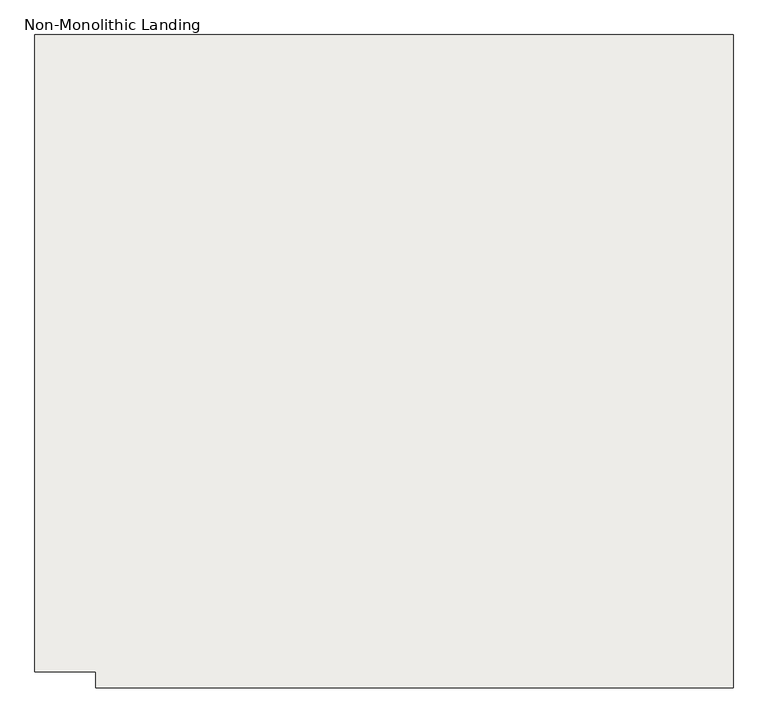
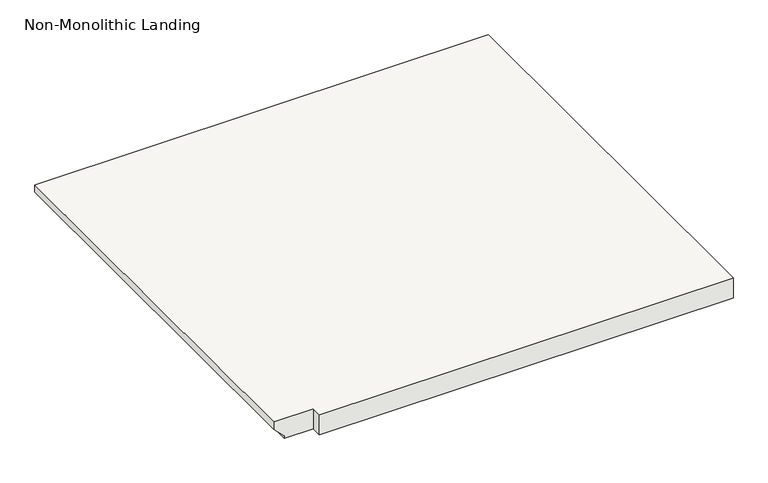
"""IFC4 building model written with IfcOpenShell, lengths in millimetres: slab geometry, Non-Monolithic Landing."""

from ifc_helpers import new_model, si_unit, origin, place, context, project, spatial, faceted_brep, source, transform, mapped, element, save


def non_monolithic_landing_4949486c(model_context):
    return source(origin(), model_context, "Body", "Brep", [
        faceted_brep([(-5053.3502524, 11195.5128362, 5772.15), (-5053.3502524, 11195.5128362, 5791.2), (-5053.3502524, 12192.4628362, 5791.2), (-5053.3502524, 12192.4628362, 5772.15), (-5027.9502524, 11195.5128362, 5746.75), (-5027.9502524, 12192.4628362, 5746.75), (-4958.1002526, 11195.5128362, 5791.2), (-4958.1002526, 11170.1128362, 5791.2), (-3961.1502526, 11170.1128362, 5791.2), (-3961.1502526, 11195.5128362, 5791.2), (-3961.1502526, 12192.4628362, 5791.2), (-5027.9502524, 11195.5128362, 5740.4), (-5027.9502524, 12192.4628362, 5740.4), (-3961.1502526, 12192.4628362, 5740.4), (-3961.1502526, 11195.5128362, 5740.4), (-3961.1502526, 11170.1128362, 5740.4), (-4958.1002526, 11170.1128362, 5740.4), (-4958.1002526, 11195.5128362, 5740.4)], [[[0, 1, 2, 3]], [[4, 0, 3, 5]], [[6, 7, 8, 9, 10, 2, 1]], [[11, 12, 13, 14, 15, 16, 17]], [[12, 11, 4, 5]], [[6, 1, 0, 4, 11, 17]], [[7, 6, 17, 16]], [[8, 7, 16, 15]], [[9, 8, 15, 14]], [[10, 9, 14, 13]], [[2, 10, 13, 12, 5, 3]]]),
    ])


if __name__ == "__main__":
    model = new_model("IFC4")
    model_context = context("Model", 3, world=origin())
    ifc_project = project(units=[si_unit("LENGTHUNIT", "METRE", prefix="MILLI")], contexts=[model_context])
    site = spatial("IfcSite", under=ifc_project)
    building = spatial("IfcBuilding", under=site)
    placement = place(None, origin())
    non_monolithic_landing_shape = non_monolithic_landing_4949486c(model_context)
    element("IfcSlab", 1, ObjectType="Non-Monolithic Landing", at=placement, inside=building, context=model_context, shape_type="MappedRepresentation", body=[
        mapped(non_monolithic_landing_shape, transform((0.0, 0.0, 0.0), x_axis=(1.0, 0.0, 0.0), y_axis=(0.0, 1.0, 0.0), z_axis=(0.0, 0.0, 1.0))),
    ])
    save(model, "model.ifc")
